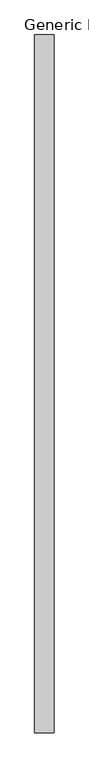
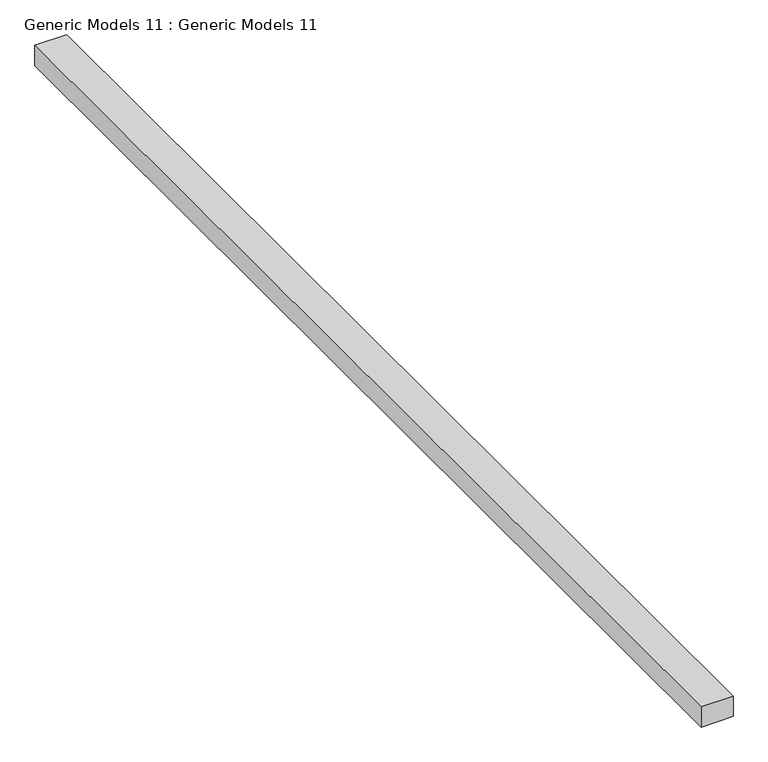
"""IFC4 building model written with IfcOpenShell, lengths in millimetres: proxy geometry, Generic Models 11 : Generic Models 11."""

from ifc_helpers import new_model, si_unit, frame, origin, place, context, project, spatial, polyline, outline, extrude, source, transform, mapped, element, save


def generic_models_11_generic_models_11_52537d9e(model_context):
    return source(origin(), model_context, "Body", "SweptSolid", [
        extrude(outline(polyline([(523.3413992, -2268.3844117), (523.3413992, -7794.7324486), (370.9413992, -7794.7324486), (370.9413992, -2268.3844117), (523.3413992, -2268.3844117)])), frame((0.0, 0.0, 6400.8), z_axis=(0.0, 0.0, 1.0), x_axis=(1.0, 0.0, 0.0)), (0.0, 0.0, 1.0), 101.6),
    ])


if __name__ == "__main__":
    model = new_model("IFC4")
    model_context = context("Model", 3, world=origin())
    ifc_project = project(units=[si_unit("LENGTHUNIT", "METRE", prefix="MILLI")], contexts=[model_context])
    site = spatial("IfcSite", under=ifc_project)
    building = spatial("IfcBuilding", under=site)
    placement = place(None, origin())
    generic_models_11_generic_models_11_shape = generic_models_11_generic_models_11_52537d9e(model_context)
    element("IfcBuildingElementProxy", 1, Name="Generic Models 11 : Generic Models 11", ObjectType="Generic Models 11 : Generic Models 11", at=placement, inside=building, context=model_context, shape_type="MappedRepresentation", body=[
        mapped(generic_models_11_generic_models_11_shape, transform((0.0, 0.0, 0.0), x_axis=(1.0, 0.0, 0.0), y_axis=(0.0, 1.0, 0.0), z_axis=(0.0, 0.0, 1.0))),
    ])
    save(model, "model.ifc")

# Revit data of these elements
# Element 1 (IfcBuildingElementProxy, "Generic Models 11 : Generic Models 11")
#   Materials on its faces: "Clad - White"
# Materials
#   "Clad - White": class "Wood", colour RGB 242 242 238, transparency 0, Cost = 0
